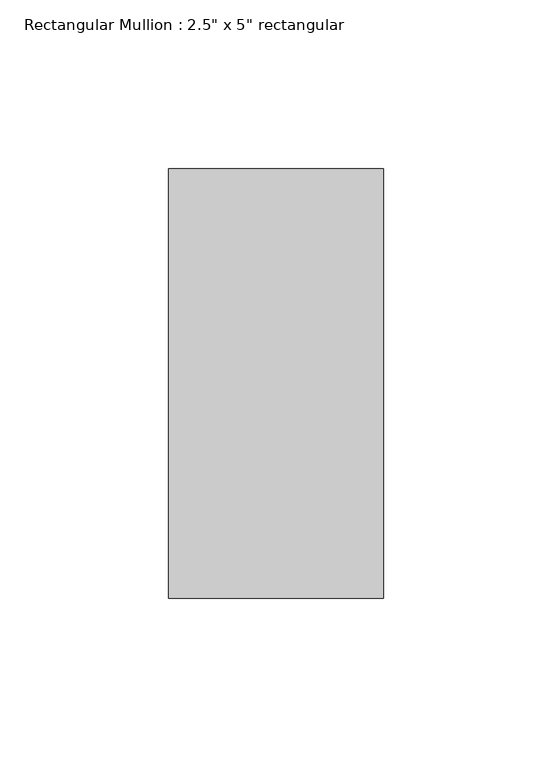
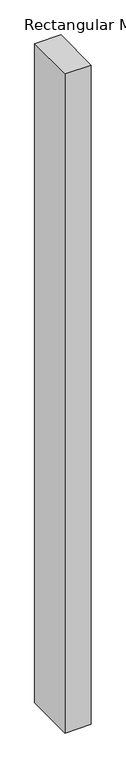
"""IFC4 building model written with IfcOpenShell, lengths in millimetres: member geometry."""

from ifc_helpers import new_model, si_unit, frame, origin, place, context, project, spatial, polyline, outline, extrude, source, transform, mapped, element, save


def member_e0a154ce(model_context):
    return source(origin(), model_context, "Body", "SweptSolid", [
        extrude(outline(polyline([(31.75, 63.5), (31.75, -63.5), (-31.75, -63.5), (-31.75, 63.5), (31.75, 63.5)])), frame((0.0, 0.0, -1687.096911), z_axis=(0.0, 0.0, 1.0), x_axis=(1.0, 0.0, 0.0)), (0.0, 0.0, 1.0), 1687.096911),
    ])


if __name__ == "__main__":
    model = new_model("IFC4")
    model_context = context("Model", 3, world=origin())
    ifc_project = project(units=[si_unit("LENGTHUNIT", "METRE", prefix="MILLI")], contexts=[model_context])
    site = spatial("IfcSite", under=ifc_project)
    building = spatial("IfcBuilding", under=site)
    placement = place(None, origin())
    member_shape = member_e0a154ce(model_context)
    element("IfcMember", 1, ObjectType="Rectangular Mullion : 2.5\" x 5\" rectangular", at=placement, inside=building, context=model_context, shape_type="MappedRepresentation", body=[
        mapped(member_shape, transform((0.0, 0.0, 0.0), x_axis=(1.0, 0.0, 0.0), y_axis=(0.0, 1.0, 0.0), z_axis=(0.0, 0.0, 1.0))),
    ])
    save(model, "model.ifc")

# Revit data of these elements
# Type "Rectangular Mullion : 2.5\" x 5\" rectangular"
#   built-in parameter 1007304 = 0.416667 (stored number, unit not read)
#   built-in parameter 1007301 = 0.104167 (stored number, unit not read)
#   built-in parameter 1007300 = 0.104167 (stored number, unit not read)
# Element 1 (IfcMember, "Rectangular Mullion : 2.5\" x 5\" rectangular")
#   Materials on its faces: "Aluminum"
# Materials
#   "Aluminum": class "Metal", colour RGB 247 247 247, transparency 0, Description = "Aluminum 6061", Cost = 0
